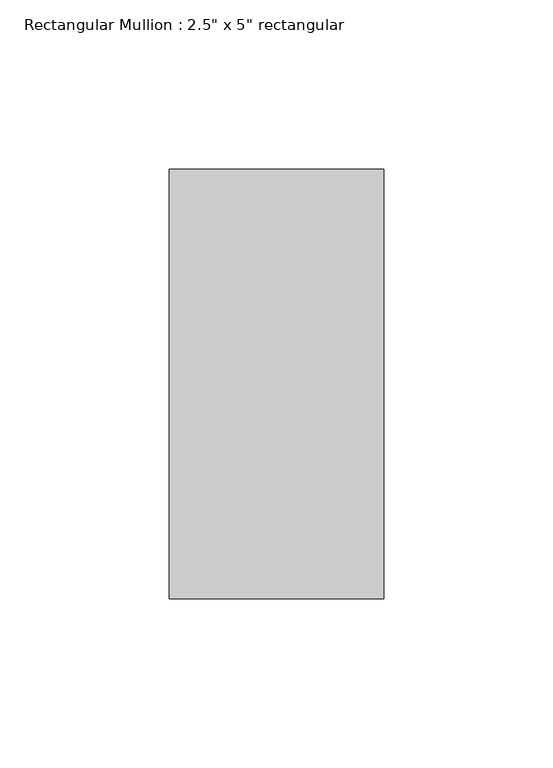
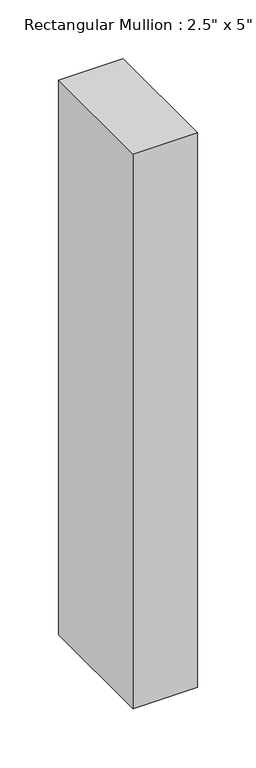
"""IFC4 building model written with IfcOpenShell, lengths in millimetres: member geometry."""

from ifc_helpers import new_model, si_unit, frame, origin, place, context, project, spatial, polyline, outline, extrude, source, transform, mapped, element, save


def member_b5e65c95(model_context):
    return source(origin(), model_context, "Body", "SweptSolid", [
        extrude(outline(polyline([(31.75, 63.5), (31.75, -63.5), (-31.75, -63.5), (-31.75, 63.5), (31.75, 63.5)])), frame((0.0, 0.0, -577.85), z_axis=(0.0, 0.0, 1.0), x_axis=(1.0, 0.0, 0.0)), (0.0, 0.0, 1.0), 577.85),
    ])


if __name__ == "__main__":
    model = new_model("IFC4")
    model_context = context("Model", 3, world=origin())
    ifc_project = project(units=[si_unit("LENGTHUNIT", "METRE", prefix="MILLI")], contexts=[model_context])
    site = spatial("IfcSite", under=ifc_project)
    building = spatial("IfcBuilding", under=site)
    placement = place(None, origin())
    member_shape = member_b5e65c95(model_context)
    element("IfcMember", 1, ObjectType="Rectangular Mullion : 2.5\" x 5\" rectangular", at=placement, inside=building, context=model_context, shape_type="MappedRepresentation", body=[
        mapped(member_shape, transform((0.0, 0.0, 0.0), x_axis=(1.0, 0.0, 0.0), y_axis=(0.0, 1.0, 0.0), z_axis=(0.0, 0.0, 1.0))),
    ])
    save(model, "model.ifc")

# Revit data of these elements
# Type "Rectangular Mullion : 2.5\" x 5\" rectangular"
#   built-in parameter 1007304 = 0.416667 (stored number, unit not read)
#   built-in parameter 1007301 = 0.104167 (stored number, unit not read)
#   built-in parameter 1007300 = 0.104167 (stored number, unit not read)
# Element 1 (IfcMember, "Rectangular Mullion : 2.5\" x 5\" rectangular")
#   Materials on its faces: "Aluminum"
# Materials
#   "Aluminum": class "Metal", colour RGB 247 247 247, transparency 0, Description = "Aluminum 6061", Cost = 0
